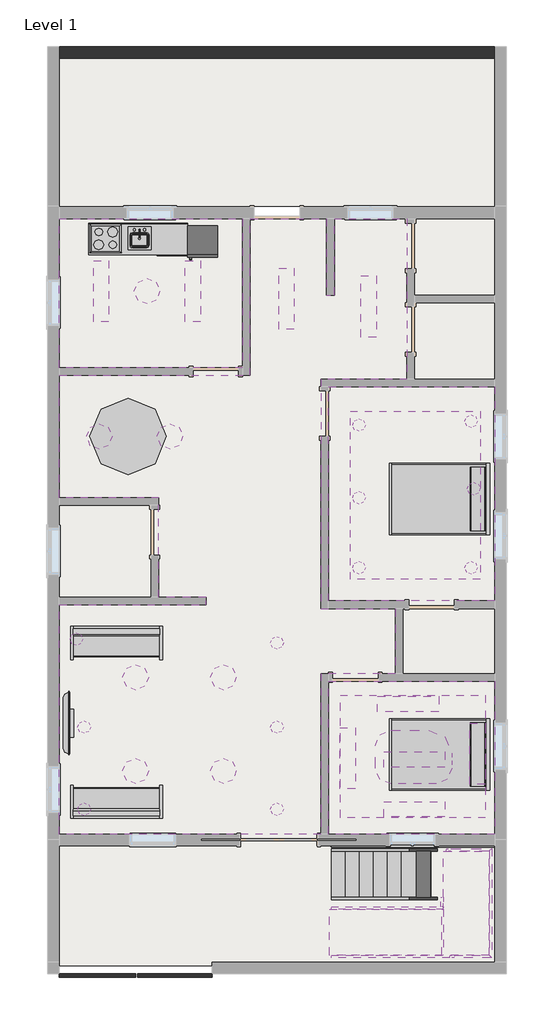
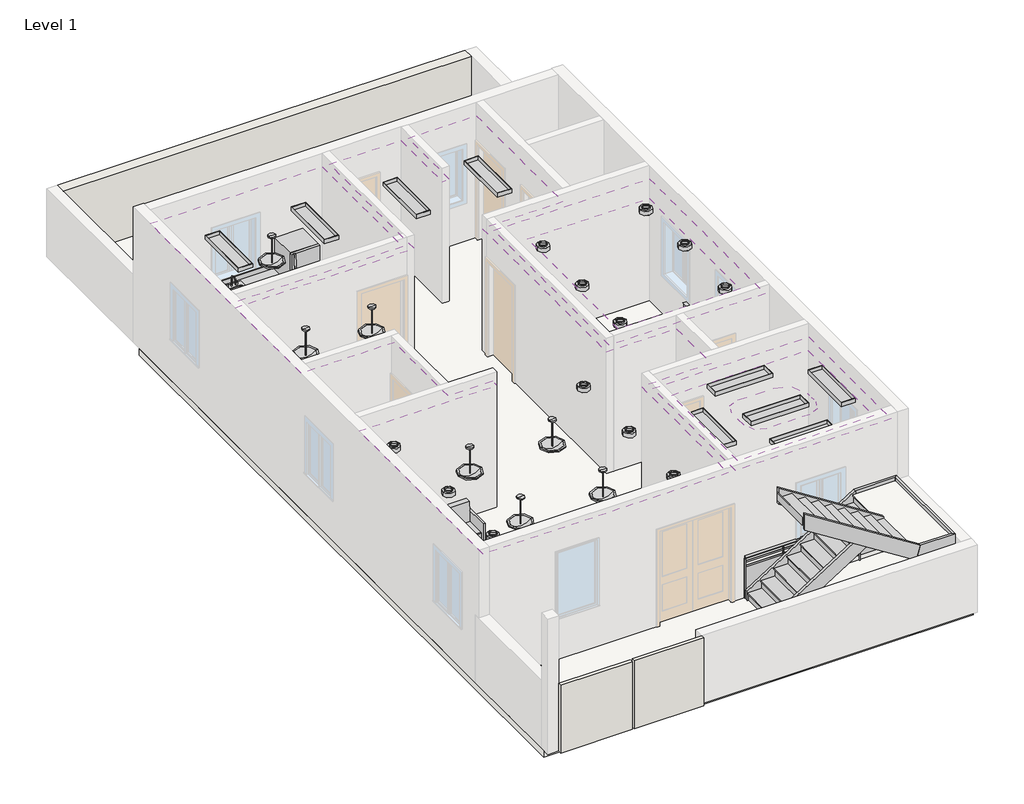
# One storey, part 2 of 2: 28 light fixtures, 8 members, 7 coverings, 7 furniture elements, 4 proxies, 3 slabs, 2 stair flights, 2 walls, 2 other elements.
# Revit data of these elements (continued)
# Element 46 (IfcLightFixture, "Pendant Light - Hemisphere : 100W - 120V") (continued)
#   Phase Created = New Construction
#   Materials on its faces: "Glass, Frosted", "Steel, Chrome Plated"
# Element 47 (IfcLightFixture, "Pendant Light - Hemisphere : 100W - 120V")
#   Mark = "20"
#   built-in parameter 1140040 = 1
#   Phase Created = New Construction
#   Materials on its faces: "Glass, Frosted", "Steel, Chrome Plated"
# Elements 48, 49, 50, 51, 52, 53, 54, 55 (IfcMember, "Stringer - 2\" Width")
#   Phase Created = New Construction
# Element 56 (IfcRailing, "Glass Panel - Bottom Fill")
#   Phase Created = New Construction
#   Materials on its faces: "Glass"
# Element 57 (IfcSlab, "6\"")
#   Height Offset From Level = 0' - 0"
#   Phase Created = New Construction
#   Materials on its faces: "FLOORING"
# Element 58 (IfcSlab, "Non-Monolithic Landing")
#   Phase Created = New Construction
# Element 59 (IfcSlab, "grass")
#   Height Offset From Level = 0' - 0"
#   Phase Created = New Construction
#   Materials on its faces: "grass"
# Elements 60, 61 (IfcStairFlight, "2\" Tread 1\" Nosing 1/4\" Riser")
#   Phase Created = New Construction
# Element 62 (IfcWall, "9\"")
#   Top Offset = 0' - 0"
#   Base Offset = 0' - 0"
#   Unconnected Height = 5' - 0"
#   wall height = 5' - 0"
#   Phase Created = New Construction
#   Base Constraint = Level 1
#   Materials on its faces: "ext walls"
# Element 63 (IfcWall, "Walls 1 : Walls 1")
#   Phase Created = New Construction
#   Materials on its faces: "Metal Deck"
# Materials
#   "Steel, Chrome Plated": class "Metal", colour RGB 17 17 17, transparency 0, Description = "Chromiuim plated steel", Cost = 0
#   "Steel, Polished": class "Metal", colour RGB 57 57 57, transparency 0, Description = "Polished steel", Cost = 0
#   "Steel, Paint Finish, Ivory, Glossy": class "Metal", colour RGB 247 247 239, transparency 0, Description = "Steel, paint finish, ivory, glossy", Cost = 0
#   "Plastic, Opaque Black": class "Plastic", colour RGB 0 0 0, transparency 0.7, Description = "Plastic, generic, opaque black", Cost = 0
#   "Cabinets": colour RGB 249 249 249, transparency 0
#   "Cabinets - Handles": class "Metal", colour RGB 57 57 57, transparency 0
#   "Default": colour RGB 127 127 127, transparency 0
#   "ceiling white": class "Generic", colour RGB 223 224 166, transparency 0, Cost = 0
#   "ceiling design": class "Generic", colour RGB 255 140 104, transparency 0, Cost = 0
#   "interior walls": class "Generic", colour RGB 114 147 63, transparency 0, Cost = 0
#   "Birch": class "Wood", colour RGB 224 178 126, transparency 0, Description = "Betula Alleghaniensis", Cost = 0
#   "Linen, White": class "Textile", colour RGB 247 247 239, transparency 0, Description = "Linen, white", Cost = 0
#   "Linen, Beige": class "Textile", colour RGB 249 239 230, transparency 0, Description = "Linen, beige", Cost = 0
#   "Cherry": class "Wood", colour RGB 226 177 128, transparency 0, Description = "Prunus Serotina", Cost = 0
#   "Pine": class "Wood", colour RGB 223 192 134, transparency 0, Description = "Pinus Echinata", Cost = 0
#   "Laminate, Linen, Matte": class "Plastic", colour RGB 249 239 230, transparency 0, Description = "Plastic Laminate - Linen, Matte", Cost = 0
#   "Steel, Paint Finish, Dark Gray, Matte": class "Metal", colour RGB 98 98 98, transparency 0, Description = "Steel, paint finish, dark gray, matte", Cost = 0
#   "Glass, White, High Luminance": class "Glass", colour RGB 249 250 249, transparency 0.8, Description = "physical material", Cost = 0
#   "Glass, Frosted": class "Glass", colour RGB 250 244 225, transparency 0.55, Description = "physical material", Cost = 0
#   "FLOORING": class "Generic", colour RGB 124 103 75, transparency 0, Cost = 0
#   "grass": class "Generic", colour RGB 127 136 91, transparency 0, Cost = 0
#   "ext walls": class "Generic", colour RGB 120 120 120, transparency 0, Cost = 0
#   "Counter Top": class "Wood", colour RGB 226 177 128, transparency 0
#   "TV - Black": colour RGB 49 49 49, transparency 0
#   "TV - Glass": colour RGB 157 157 157, transparency 0.9
#   "TV - Screen": colour RGB 0 0 0, transparency 0
#   "Glass": class "Glass", colour RGB 0 128 192, transparency 0.75, Description = "Soda Lime Glass", Cost = 0
#   "Metal Deck": class "Metal", colour RGB 83 83 80, transparency 0, Description = "Steel, mill finish", Cost = 0
